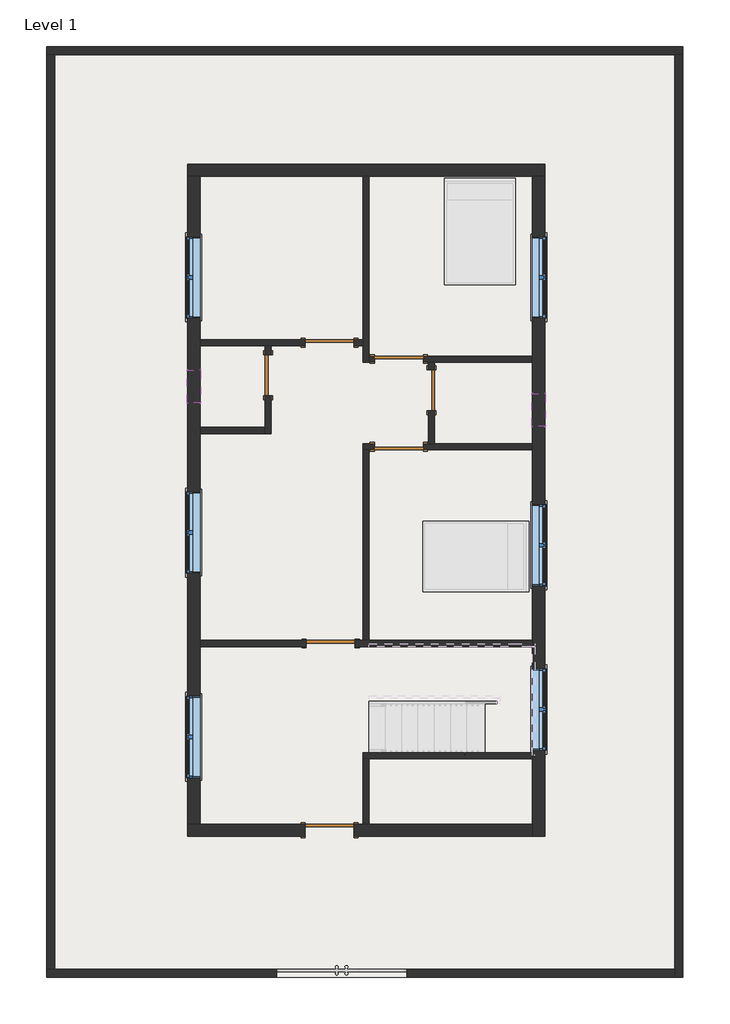
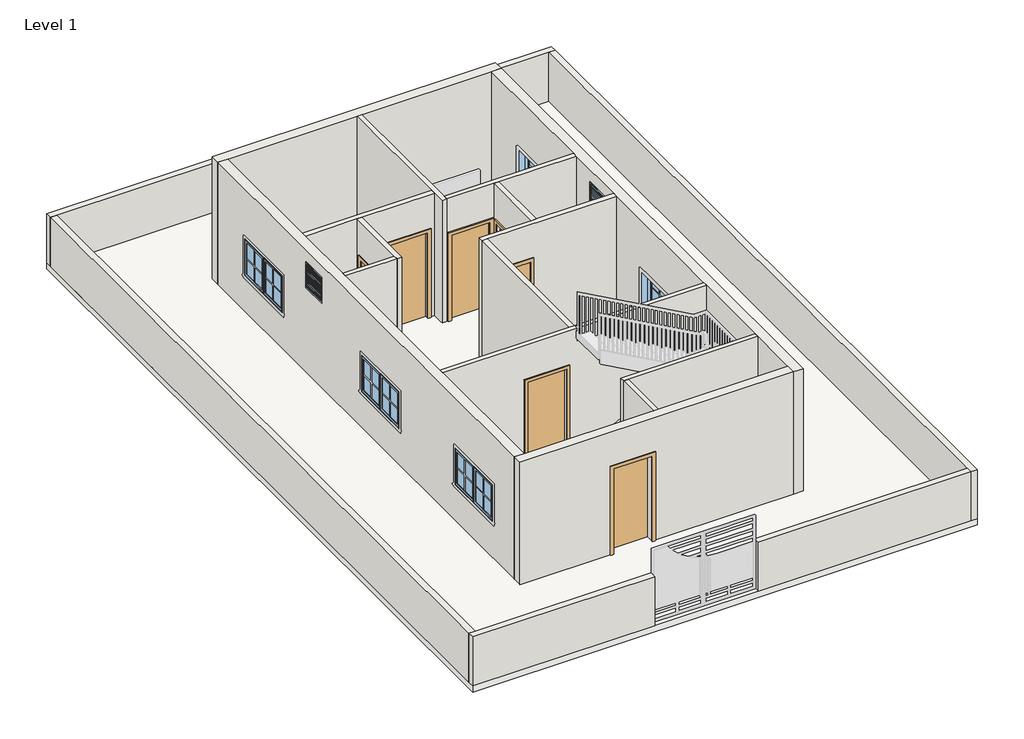
# One storey, part 1 of 3: 20 walls, 8 windows, 7 doors, 1 slab.
"""IFC4 building model written with IfcOpenShell, lengths in millimetres."""

from ifc_helpers import new_model, si_unit, frame, origin, origin_with_axes, place, context, project, spatial, polyline, outline, extrude, faceted_brep, transform, mapped, element, save
from components import door_78caadf7, door_214872d5, single_flush_door_3_e5f9f3c4, single_flush_door_3_305aa2a5, single_flush_door_3_0ca8825f, window_casement_double_win_5_c1d95f0f, window_f2d8fef0

model = new_model("IFC4")

# Units and contexts
model_context = context("Model", 3, world=origin())
ifc_project = project(units=[si_unit("LENGTHUNIT", "METRE", prefix="MILLI")], contexts=[model_context])

# Site, building, storey
site = spatial("IfcSite", under=ifc_project)
building = spatial("IfcBuilding", under=site)
storey = spatial("IfcBuildingStorey", under=building, Name="Level 1", Elevation=0.0)

# Doors
placement = place(None, origin())
door_shape = door_78caadf7(model_context)
element("IfcDoor", 1, ObjectType="Single-Flush : 2'6\"", at=placement, inside=storey, context=model_context, shape_type="MappedRepresentation", body=[
    mapped(door_shape, transform((-35.92188, 1946.24131, 0.0), x_axis=(0.0, 1.0, 0.0), y_axis=(-1.0, 0.0, 0.0), z_axis=(0.0, 0.0, 1.0))),
])
door_2_shape = door_214872d5(model_context)
element("IfcDoor", 2, ObjectType="Single-Flush : 2'6\"", at=placement, inside=storey, context=model_context, shape_type="MappedRepresentation", body=[
    mapped(door_2_shape, transform((-3083.92188, 2225.64131, 0.0), x_axis=(0.0, 1.0, 0.0), y_axis=(-1.0, 0.0, 0.0), z_axis=(0.0, 0.0, 1.0))),
])
single_flush_door_3_shape = single_flush_door_3_e5f9f3c4(model_context)
element("IfcDoor", 3, ObjectType="Single-Flush : DOOR 3'", at=placement, inside=storey, context=model_context, shape_type="MappedRepresentation", body=[
    mapped(single_flush_door_3_shape, transform((-1940.92188, 2835.24131, 0.0), x_axis=(1.0, 0.0, 0.0), y_axis=(0.0, 1.0, 0.0), z_axis=(0.0, 0.0, 1.0))),
])
element("IfcDoor", 4, ObjectType="Single-Flush : DOOR 3'", at=placement, inside=storey, context=model_context, shape_type="MappedRepresentation", body=[
    mapped(single_flush_door_3_shape, transform((-645.52188, 892.14131, 0.0), x_axis=(-1.0, 0.0, 0.0), y_axis=(0.0, -1.0, 0.0), z_axis=(0.0, 0.0, 1.0))),
])
element("IfcDoor", 5, ObjectType="Single-Flush : DOOR 3'", at=placement, inside=storey, context=model_context, shape_type="MappedRepresentation", body=[
    mapped(single_flush_door_3_shape, transform((-1915.52188, -2778.15869, 0.0), x_axis=(1.0, 0.0, 0.0), y_axis=(0.0, 1.0, 0.0), z_axis=(0.0, 0.0, 1.0))),
])
single_flush_door_3_2_shape = single_flush_door_3_305aa2a5(model_context)
element("IfcDoor", 6, ObjectType="Single-Flush : DOOR 3'", at=placement, inside=storey, context=model_context, shape_type="MappedRepresentation", body=[
    mapped(single_flush_door_3_2_shape, transform((-645.52188, 2530.44131, 0.0), x_axis=(-1.0, 0.0, 0.0), y_axis=(0.0, -1.0, 0.0), z_axis=(0.0, 0.0, 1.0))),
])
single_flush_door_3_3_shape = single_flush_door_3_0ca8825f(model_context)
element("IfcDoor", 7, ObjectType="Single-Flush : DOOR 3'", at=placement, inside=storey, context=model_context, shape_type="MappedRepresentation", body=[
    mapped(single_flush_door_3_3_shape, transform((-1940.92188, -6264.30869, 0.0), x_axis=(1.0, 0.0, 0.0), y_axis=(0.0, 1.0, 0.0), z_axis=(0.0, 0.0, 1.0))),
])

# Slab
element("IfcSlab", 8, ObjectType="FLOOR 6\"", at=placement, inside=storey, context=model_context, shape_type="SweptSolid", body=[
    extrude(outline(polyline([(4662.9483709, 8363.0499713), (4662.9483709, -9010.5500287), (-7224.2516291, -9010.5500287), (-7224.2516291, 8363.0499713), (4662.9483709, 8363.0499713)])), frame((0.0, 0.0, -152.4), z_axis=(0.0, 0.0, 1.0), x_axis=(1.0, 0.0, 0.0)), (0.0, 0.0, 1.0), 152.4),
])

# Walls
element("IfcWall", 9, ObjectType="CMD 6\"", at=placement, inside=storey, context=model_context, shape_type="Brep", body=[
    faceted_brep([(-7224.2516291, 8210.6499713, 0.0), (-7071.8516291, 8210.6499713, 0.0), (4510.5483709, 8210.6499713, 0.0), (4662.9483709, 8210.6499713, 0.0), (4662.9483709, 8210.6499713, 1219.2), (4510.5483709, 8210.6499713, 1219.2), (-7071.8516291, 8210.6499713, 1219.2), (-7224.2516291, 8210.6499713, 1219.2), (-7224.2516291, 8363.0499713, 0.0), (-7224.2516291, 8363.0499713, 1219.2), (4662.9483709, 8363.0499713, 1219.2), (4662.9483709, 8363.0499713, 0.0)], [[[0, 1, 2, 3, 4, 5, 6, 7]], [[8, 9, 10, 11]], [[3, 2, 1, 0, 8, 11]], [[7, 6, 5, 4, 10, 9]], [[4, 3, 11, 10]], [[0, 7, 9, 8]]]),
])
element("IfcWall", 10, ObjectType="CMD 6\"", at=placement, inside=storey, context=model_context, shape_type="Brep", body=[
    faceted_brep([(4510.5483709, 8210.6499713, 0.0), (4510.5483709, -8858.1500287, 0.0), (4510.5483709, -9010.5500287, 0.0), (4510.5483709, -9010.5500287, 1219.2), (4510.5483709, -8858.1500287, 1219.2), (4510.5483709, 8210.6499713, 1219.2), (4662.9483709, 8210.6499713, 0.0), (4662.9483709, 8210.6499713, 1219.2), (4662.9483709, -9010.5500287, 1219.2), (4662.9483709, -9010.5500287, 0.0)], [[[0, 1, 2, 3, 4, 5]], [[6, 7, 8, 9]], [[2, 1, 0, 6, 9]], [[5, 4, 3, 8, 7]], [[0, 5, 7, 6]], [[3, 2, 9, 8]]]),
])
element("IfcWall", 11, ObjectType="CMD 6\"", at=placement, inside=storey, context=model_context, shape_type="SweptSolid", body=[
    extrude(outline(polyline([(-493.12188, -8858.1500287), (4510.5483709, -8858.1500287), (4510.5483709, -9010.5500287), (-493.12188, -9010.5500287), (-493.12188, -8858.1500287)])), origin_with_axes(), (0.0, 0.0, 1.0), 1219.2),
])
element("IfcWall", 12, ObjectType="CMD 6\"", at=placement, inside=storey, context=model_context, shape_type="SweptSolid", body=[
    extrude(outline(polyline([(-7071.8516291, 8210.6499713), (-7071.8516291, -8858.1500287), (-7224.2516291, -8858.1500287), (-7224.2516291, 8210.6499713), (-7071.8516291, 8210.6499713)])), origin_with_axes(), (0.0, 0.0, 1.0), 1219.2),
])
element("IfcWall", 13, ObjectType="CMD 6\"", at=placement, inside=storey, context=model_context, shape_type="Brep", body=[
    faceted_brep([(-2931.52188, -8858.1500287, 0.0), (-7071.8516291, -8858.1500287, 0.0), (-7224.2516291, -8858.1500287, 0.0), (-7224.2516291, -8858.1500287, 1219.2), (-7071.8516291, -8858.1500287, 1219.2), (-2931.52188, -8858.1500287, 1219.2), (-2931.52188, -9010.5500287, 0.0), (-2931.52188, -9010.5500287, 1219.2), (-7224.2516291, -9010.5500287, 1219.2), (-7224.2516291, -9010.5500287, 0.0)], [[[0, 1, 2, 3, 4, 5]], [[6, 7, 8, 9]], [[2, 1, 0, 6, 9]], [[5, 4, 3, 8, 7]], [[0, 5, 7, 6]], [[3, 2, 9, 8]]]),
])
element("IfcWall", 14, ObjectType="WALL 4.5'", at=placement, inside=storey, context=model_context, shape_type="Brep", body=[
    faceted_brep([(-1312.27188, 5940.39131, 0.0), (-1312.27188, 2892.39131, 0.0), (-1312.27188, 2778.09131, 0.0), (-1312.27188, 2473.29131, 0.0), (-1312.27188, 2473.29131, 3048.0), (-1312.27188, 2778.09131, 3048.0), (-1312.27188, 2892.39131, 3048.0), (-1312.27188, 5940.39131, 3048.0), (-1197.97188, 5940.39131, 0.0), (-1197.97188, 5940.39131, 3048.0), (-1197.97188, 2587.59131, 3048.0), (-1197.97188, 2473.29131, 3048.0), (-1197.97188, 2473.29131, 0.0), (-1197.97188, 2587.59131, 0.0)], [[[0, 1, 2, 3, 4, 5, 6, 7]], [[8, 9, 10, 11, 12, 13]], [[3, 2, 1, 0, 8, 13, 12]], [[0, 7, 9, 8]], [[4, 3, 12, 11]], [[7, 6, 5, 4, 11, 10, 9]]]),
])
element("IfcWall", 15, ObjectType="WALL 4.5'", at=placement, inside=storey, context=model_context, shape_type="Brep", body=[
    faceted_brep([(-1197.97188, 2473.29131, 0.0), (-1102.72188, 2473.29131, 0.0), (-1102.72188, 2473.29131, 2133.6), (-188.32188, 2473.29131, 2133.6), (-188.32188, 2473.29131, 0.0), (-93.07188, 2473.29131, 0.0), (21.22812, 2473.29131, 0.0), (1850.02812, 2473.29131, 0.0), (1850.02812, 2473.29131, 3048.0), (21.22812, 2473.29131, 3048.0), (-93.07188, 2473.29131, 3048.0), (-1197.97188, 2473.29131, 3048.0), (-1102.72188, 2587.59131, 2133.6), (-1102.72188, 2587.59131, 0.0), (-1197.97188, 2587.59131, 0.0), (-1197.97188, 2587.59131, 3048.0), (1850.02812, 2587.59131, 3048.0), (1850.02812, 2587.59131, 0.0), (-188.32188, 2587.59131, 0.0), (-188.32188, 2587.59131, 2133.6)], [[[0, 1, 2, 3, 4, 5, 6, 7, 8, 9, 10, 11]], [[12, 13, 14, 15, 16, 17, 18, 19]], [[18, 17, 7, 6, 5, 4]], [[14, 13, 1, 0]], [[0, 11, 15, 14]], [[8, 7, 17, 16]], [[2, 1, 13, 12]], [[3, 2, 12, 19]], [[4, 3, 19, 18]], [[11, 10, 9, 8, 16, 15]]]),
])
element("IfcWall", 16, ObjectType="WALL 4.5'", at=placement, inside=storey, context=model_context, shape_type="Brep", body=[
    faceted_brep([(-1312.27188, 2892.39131, 0.0), (-1483.72188, 2892.39131, 0.0), (-1483.72188, 2892.39131, 2133.6), (-2398.12188, 2892.39131, 2133.6), (-2398.12188, 2892.39131, 0.0), (-4360.27188, 2892.39131, 0.0), (-4360.27188, 2892.39131, 3048.0), (-1312.27188, 2892.39131, 3048.0), (-1483.72188, 2778.09131, 2133.6), (-1483.72188, 2778.09131, 0.0), (-1312.27188, 2778.09131, 0.0), (-1312.27188, 2778.09131, 3048.0), (-3026.77188, 2778.09131, 3048.0), (-3141.07188, 2778.09131, 3048.0), (-4360.27188, 2778.09131, 3048.0), (-4360.27188, 2778.09131, 0.0), (-3141.07188, 2778.09131, 0.0), (-3026.77188, 2778.09131, 0.0), (-2398.12188, 2778.09131, 0.0), (-2398.12188, 2778.09131, 2133.6)], [[[0, 1, 2, 3, 4, 5, 6, 7]], [[8, 9, 10, 11, 12, 13, 14, 15, 16, 17, 18, 19]], [[10, 9, 1, 0]], [[18, 17, 16, 15, 5, 4]], [[6, 5, 15, 14]], [[0, 7, 11, 10]], [[2, 1, 9, 8]], [[3, 2, 8, 19]], [[4, 3, 19, 18]], [[7, 6, 14, 13, 12, 11]]]),
])
element("IfcWall", 17, ObjectType="WALL 4.5'", at=placement, inside=storey, context=model_context, shape_type="Brep", body=[
    faceted_brep([(-3141.07188, 2778.09131, 0.0), (-3141.07188, 2606.64131, 0.0), (-3141.07188, 2606.64131, 2133.6), (-3141.07188, 1844.64131, 2133.6), (-3141.07188, 1844.64131, 0.0), (-3141.07188, 1254.09131, 0.0), (-3141.07188, 1139.79131, 0.0), (-3141.07188, 1139.79131, 3048.0), (-3141.07188, 1254.09131, 3048.0), (-3141.07188, 2778.09131, 3048.0), (-3026.77188, 2606.64131, 2133.6), (-3026.77188, 2606.64131, 0.0), (-3026.77188, 2778.09131, 0.0), (-3026.77188, 2778.09131, 3048.0), (-3026.77188, 1139.79131, 3048.0), (-3026.77188, 1139.79131, 0.0), (-3026.77188, 1844.64131, 0.0), (-3026.77188, 1844.64131, 2133.6)], [[[0, 1, 2, 3, 4, 5, 6, 7, 8, 9]], [[10, 11, 12, 13, 14, 15, 16, 17]], [[16, 15, 6, 5, 4]], [[12, 11, 1, 0]], [[0, 9, 13, 12]], [[7, 6, 15, 14]], [[2, 1, 11, 10]], [[3, 2, 10, 17]], [[4, 3, 17, 16]], [[9, 8, 7, 14, 13]]]),
])
element("IfcWall", 18, ObjectType="WALL 4.5'", at=placement, inside=storey, context=model_context, shape_type="SweptSolid", body=[
    extrude(outline(polyline([(-4360.27188, 1254.09131), (-3141.07188, 1254.09131), (-3141.07188, 1139.79131), (-4360.27188, 1139.79131), (-4360.27188, 1254.09131)])), origin_with_axes(), (0.0, 0.0, 1.0), 3048.0),
])
element("IfcWall", 19, ObjectType="WALL 4.5'", at=placement, inside=storey, context=model_context, shape_type="SweptSolid", body=[
    extrude(outline(polyline([(2473.29131, 0.0), (2327.24131, 0.0), (2327.24131, 2133.6), (1565.24131, 2133.6), (1565.24131, 0.0), (949.29131, 0.0), (949.29131, 3048.0), (2473.29131, 3048.0), (2473.29131, 0.0)])), frame((-93.07188, 0.0, 0.0), z_axis=(1.0, 0.0, 0.0), x_axis=(0.0, 1.0, 0.0)), (0.0, 0.0, 1.0), 114.3),
])
element("IfcWall", 20, ObjectType="WALL 4.5'", at=placement, inside=storey, context=model_context, shape_type="Brep", body=[
    faceted_brep([(-1102.72188, 949.29131, 2133.6), (-1102.72188, 949.29131, 0.0), (-1312.27188, 949.29131, 0.0), (-1312.27188, 949.29131, 3048.0), (-93.07188, 949.29131, 3048.0), (21.22812, 949.29131, 3048.0), (1850.02812, 949.29131, 3048.0), (1850.02812, 949.29131, 0.0), (21.22812, 949.29131, 0.0), (-93.07188, 949.29131, 0.0), (-188.32188, 949.29131, 0.0), (-188.32188, 949.29131, 2133.6), (-1312.27188, 834.99131, 0.0), (-1197.97188, 834.99131, 0.0), (-1102.72188, 834.99131, 0.0), (-1102.72188, 834.99131, 2133.6), (-188.32188, 834.99131, 2133.6), (-188.32188, 834.99131, 0.0), (1850.02812, 834.99131, 0.0), (1850.02812, 834.99131, 3048.0), (-1197.97188, 834.99131, 3048.0), (-1312.27188, 834.99131, 3048.0)], [[[0, 1, 2, 3, 4, 5, 6, 7, 8, 9, 10, 11]], [[12, 13, 14, 15, 16, 17, 18, 19, 20, 21]], [[2, 1, 14, 13, 12]], [[10, 9, 8, 7, 18, 17]], [[7, 6, 19, 18]], [[3, 2, 12, 21]], [[15, 14, 1, 0]], [[16, 15, 0, 11]], [[17, 16, 11, 10]], [[6, 5, 4, 3, 21, 20, 19]]]),
])
element("IfcWall", 21, ObjectType="WALL 4.5'", at=placement, inside=storey, context=model_context, shape_type="SweptSolid", body=[
    extrude(outline(polyline([(-1312.27188, -2721.00869), (-1312.27188, 834.99131), (-1197.97188, 834.99131), (-1197.97188, -2721.00869), (-1312.27188, -2721.00869)])), origin_with_axes(), (0.0, 0.0, 1.0), 3048.0),
])
element("IfcWall", 22, ObjectType="WALL 4.5'", at=placement, inside=storey, context=model_context, shape_type="Brep", body=[
    faceted_brep([(1850.02812, -2721.00869, 0.0), (-1197.97188, -2721.00869, 0.0), (-1312.27188, -2721.00869, 0.0), (-1458.32188, -2721.00869, 0.0), (-1458.32188, -2721.00869, 2133.6), (-2372.72188, -2721.00869, 2133.6), (-2372.72188, -2721.00869, 0.0), (-4360.27188, -2721.00869, 0.0), (-4360.27188, -2721.00869, 3048.0), (-1312.27188, -2721.00869, 3048.0), (-1197.97188, -2721.00869, 3048.0), (1850.02812, -2721.00869, 3048.0), (-1458.32188, -2835.30869, 2133.6), (-1458.32188, -2835.30869, 0.0), (1850.02812, -2835.30869, 0.0), (1850.02812, -2835.30869, 3048.0), (-4360.27188, -2835.30869, 3048.0), (-4360.27188, -2835.30869, 0.0), (-2372.72188, -2835.30869, 0.0), (-2372.72188, -2835.30869, 2133.6)], [[[0, 1, 2, 3, 4, 5, 6, 7, 8, 9, 10, 11]], [[12, 13, 14, 15, 16, 17, 18, 19]], [[18, 17, 7, 6]], [[14, 13, 3, 2, 1, 0]], [[0, 11, 15, 14]], [[8, 7, 17, 16]], [[4, 3, 13, 12]], [[5, 4, 12, 19]], [[6, 5, 19, 18]], [[11, 10, 9, 8, 16, 15]]]),
])
element("IfcWall", 23, ObjectType="WALL 4.5'", at=placement, inside=storey, context=model_context, shape_type="Brep", body=[
    faceted_brep([(1850.02812, -4816.50869, 0.0), (-1312.27188, -4816.50869, 0.0), (-1312.27188, -4816.50869, 3048.0), (1850.02812, -4816.50869, 3048.0), (1850.02812, -4930.80869, 0.0), (1850.02812, -4930.80869, 3048.0), (-1197.97188, -4930.80869, 3048.0), (-1312.27188, -4930.80869, 3048.0), (-1312.27188, -4930.80869, 0.0), (-1197.97188, -4930.80869, 0.0)], [[[0, 1, 2, 3]], [[4, 5, 6, 7, 8, 9]], [[1, 0, 4, 9, 8]], [[0, 3, 5, 4]], [[2, 1, 8, 7]], [[3, 2, 7, 6, 5]]]),
])
element("IfcWall", 24, ObjectType="WALL 4.5'", at=placement, inside=storey, context=model_context, shape_type="SweptSolid", body=[
    extrude(outline(polyline([(-1312.27188, -6150.00869), (-1312.27188, -4930.80869), (-1197.97188, -4930.80869), (-1197.97188, -6150.00869), (-1312.27188, -6150.00869)])), origin_with_axes(), (0.0, 0.0, 1.0), 3048.0),
])
element("IfcWall", 25, ObjectType="WALL 9\"", at=placement, inside=storey, context=model_context, shape_type="Brep", body=[
    faceted_brep([(-4588.87188, 5940.39131, 0.0), (-4360.27188, 5940.39131, 0.0), (-1312.27188, 5940.39131, 0.0), (-1197.97188, 5940.39131, 0.0), (1850.02812, 5940.39131, 0.0), (2078.62812, 5940.39131, 0.0), (2078.62812, 5940.39131, 3048.0), (1850.02812, 5940.39131, 3048.0), (-1197.97188, 5940.39131, 3048.0), (-1312.27188, 5940.39131, 3048.0), (-4360.27188, 5940.39131, 3048.0), (-4588.87188, 5940.39131, 3048.0), (-4588.87188, 6168.99131, 0.0), (-4588.87188, 6168.99131, 3048.0), (2078.62812, 6168.99131, 3048.0), (2078.62812, 6168.99131, 0.0)], [[[0, 1, 2, 3, 4, 5, 6, 7, 8, 9, 10, 11]], [[12, 13, 14, 15]], [[5, 4, 3, 2, 1, 0, 12, 15]], [[6, 5, 15, 14]], [[0, 11, 13, 12]], [[11, 10, 9, 8, 7, 6, 14, 13]]]),
])
element("IfcWall", 26, ObjectType="WALL 9\"", at=placement, inside=storey, context=model_context, shape_type="Brep", body=[
    faceted_brep([(1850.02812, 5940.39131, 0.0), (1850.02812, 2587.59131, 0.0), (1850.02812, 2473.29131, 0.0), (1850.02812, 949.29131, 0.0), (1850.02812, 834.99131, 0.0), (1850.02812, -2721.00869, 0.0), (1850.02812, -2835.30869, 0.0), (1850.02812, -4816.50869, 0.0), (1850.02812, -4930.80869, 0.0), (1850.02812, -6150.00869, 0.0), (1850.02812, -6378.60869, 0.0), (1850.02812, -6378.60869, 3048.0), (1850.02812, -6150.00869, 3048.0), (1850.02812, -4930.80869, 3048.0), (1850.02812, -4816.50869, 3048.0), (1850.02812, -2835.30869, 3048.0), (1850.02812, -2721.00869, 3048.0), (1850.02812, 834.99131, 3048.0), (1850.02812, 949.29131, 3048.0), (1850.02812, 2473.29131, 3048.0), (1850.02812, 2587.59131, 3048.0), (1850.02812, 5940.39131, 3048.0), (1850.02812, -4772.05869, 1828.8), (1850.02812, -4772.05869, 914.4), (1850.02812, -3248.05869, 914.4), (1850.02812, -3248.05869, 1828.8), (1850.02812, 3292.44131, 1828.8), (1850.02812, 3292.44131, 914.4), (1850.02812, 4816.44131, 914.4), (1850.02812, 4816.44131, 1828.8), (1850.02812, -1705.00869, 1828.8), (1850.02812, -1705.00869, 914.4), (1850.02812, -181.00869, 914.4), (1850.02812, -181.00869, 1828.8), (1850.02812, 1273.14131, 2743.2), (1850.02812, 1273.14131, 2133.6), (1850.02812, 1882.74131, 2133.6), (1850.02812, 1882.74131, 2743.2), (2078.62812, 5940.39131, 0.0), (2078.62812, 5940.39131, 3048.0), (2078.62812, -6378.60869, 3048.0), (2078.62812, -6378.60869, 0.0), (2078.62812, -4772.05869, 1828.8), (2078.62812, -3248.05869, 1828.8), (2078.62812, -3248.05869, 914.4), (2078.62812, -4772.05869, 914.4), (2078.62812, 3292.44131, 1828.8), (2078.62812, 4816.44131, 1828.8), (2078.62812, 4816.44131, 914.4), (2078.62812, 3292.44131, 914.4), (2078.62812, -1705.00869, 1828.8), (2078.62812, -181.00869, 1828.8), (2078.62812, -181.00869, 914.4), (2078.62812, -1705.00869, 914.4), (2078.62812, 1273.14131, 2743.2), (2078.62812, 1882.74131, 2743.2), (2078.62812, 1882.74131, 2133.6), (2078.62812, 1273.14131, 2133.6)], [[[0, 1, 2, 3, 4, 5, 6, 7, 8, 9, 10, 11, 12, 13, 14, 15, 16, 17, 18, 19, 20, 21], [22, 23, 24, 25], [26, 27, 28, 29], [30, 31, 32, 33], [34, 35, 36, 37]], [[38, 39, 40, 41], [42, 43, 44, 45], [46, 47, 48, 49], [50, 51, 52, 53], [54, 55, 56, 57]], [[10, 9, 8, 7, 6, 5, 4, 3, 2, 1, 0, 38, 41]], [[0, 21, 39, 38]], [[11, 10, 41, 40]], [[23, 22, 42, 45]], [[24, 23, 45, 44]], [[25, 24, 44, 43]], [[22, 25, 43, 42]], [[27, 26, 46, 49]], [[28, 27, 49, 48]], [[29, 28, 48, 47]], [[26, 29, 47, 46]], [[31, 30, 50, 53]], [[32, 31, 53, 52]], [[33, 32, 52, 51]], [[30, 33, 51, 50]], [[35, 34, 54, 57]], [[36, 35, 57, 56]], [[37, 36, 56, 55]], [[34, 37, 55, 54]], [[21, 20, 19, 18, 17, 16, 15, 14, 13, 12, 11, 40, 39]]]),
])
element("IfcWall", 27, ObjectType="WALL 9\"", at=placement, inside=storey, context=model_context, shape_type="Brep", body=[
    faceted_brep([(1850.02812, -6150.00869, 0.0), (-1197.97188, -6150.00869, 0.0), (-1312.27188, -6150.00869, 0.0), (-1483.72188, -6150.00869, 0.0), (-1483.72188, -6150.00869, 2133.6), (-2398.12188, -6150.00869, 2133.6), (-2398.12188, -6150.00869, 0.0), (-4360.27188, -6150.00869, 0.0), (-4588.87188, -6150.00869, 0.0), (-4588.87188, -6150.00869, 3048.0), (-4360.27188, -6150.00869, 3048.0), (-1312.27188, -6150.00869, 3048.0), (-1197.97188, -6150.00869, 3048.0), (1850.02812, -6150.00869, 3048.0), (-1483.72188, -6378.60869, 2133.6), (-1483.72188, -6378.60869, 0.0), (1850.02812, -6378.60869, 0.0), (1850.02812, -6378.60869, 3048.0), (-4588.87188, -6378.60869, 3048.0), (-4588.87188, -6378.60869, 0.0), (-2398.12188, -6378.60869, 0.0), (-2398.12188, -6378.60869, 2133.6)], [[[0, 1, 2, 3, 4, 5, 6, 7, 8, 9, 10, 11, 12, 13]], [[14, 15, 16, 17, 18, 19, 20, 21]], [[20, 19, 8, 7, 6]], [[16, 15, 3, 2, 1, 0]], [[0, 13, 17, 16]], [[9, 8, 19, 18]], [[4, 3, 15, 14]], [[5, 4, 14, 21]], [[6, 5, 21, 20]], [[13, 12, 11, 10, 9, 18, 17]]]),
])
element("IfcWall", 28, ObjectType="WALL 9\"", at=placement, inside=storey, context=model_context, shape_type="Brep", body=[
    faceted_brep([(-4360.27188, -6150.00869, 0.0), (-4360.27188, -2835.30869, 0.0), (-4360.27188, -2721.00869, 0.0), (-4360.27188, 1139.79131, 0.0), (-4360.27188, 1254.09131, 0.0), (-4360.27188, 2778.09131, 0.0), (-4360.27188, 2892.39131, 0.0), (-4360.27188, 5940.39131, 0.0), (-4360.27188, 5940.39131, 3048.0), (-4360.27188, 2892.39131, 3048.0), (-4360.27188, 2778.09131, 3048.0), (-4360.27188, 1254.09131, 3048.0), (-4360.27188, 1139.79131, 3048.0), (-4360.27188, -2721.00869, 3048.0), (-4360.27188, -2835.30869, 3048.0), (-4360.27188, -6150.00869, 3048.0), (-4360.27188, 4816.44131, 1828.8), (-4360.27188, 4816.44131, 914.4), (-4360.27188, 3292.44131, 914.4), (-4360.27188, 3292.44131, 1828.8), (-4360.27188, 53.94131, 1828.8), (-4360.27188, 53.94131, 914.4), (-4360.27188, -1470.05869, 914.4), (-4360.27188, -1470.05869, 1828.8), (-4360.27188, -3759.23369, 1828.8), (-4360.27188, -3759.23369, 914.4), (-4360.27188, -5283.23369, 914.4), (-4360.27188, -5283.23369, 1828.8), (-4360.27188, 1711.29131, 2743.2), (-4360.27188, 2320.89131, 2743.2), (-4360.27188, 2320.89131, 2133.6), (-4360.27188, 1711.29131, 2133.6), (-4588.87188, -6150.00869, 0.0), (-4588.87188, -6150.00869, 3048.0), (-4588.87188, 5940.39131, 3048.0), (-4588.87188, 5940.39131, 0.0), (-4588.87188, 4816.44131, 1828.8), (-4588.87188, 3292.44131, 1828.8), (-4588.87188, 3292.44131, 914.4), (-4588.87188, 4816.44131, 914.4), (-4588.87188, 53.94131, 1828.8), (-4588.87188, -1470.05869, 1828.8), (-4588.87188, -1470.05869, 914.4), (-4588.87188, 53.94131, 914.4), (-4588.87188, -3759.23369, 1828.8), (-4588.87188, -5283.23369, 1828.8), (-4588.87188, -5283.23369, 914.4), (-4588.87188, -3759.23369, 914.4), (-4588.87188, 1711.29131, 2743.2), (-4588.87188, 1711.29131, 2133.6), (-4588.87188, 2320.89131, 2133.6), (-4588.87188, 2320.89131, 2743.2)], [[[0, 1, 2, 3, 4, 5, 6, 7, 8, 9, 10, 11, 12, 13, 14, 15], [16, 17, 18, 19], [20, 21, 22, 23], [24, 25, 26, 27], [28, 29, 30, 31]], [[32, 33, 34, 35], [36, 37, 38, 39], [40, 41, 42, 43], [44, 45, 46, 47], [48, 49, 50, 51]], [[7, 6, 5, 4, 3, 2, 1, 0, 32, 35]], [[8, 7, 35, 34]], [[0, 15, 33, 32]], [[17, 16, 36, 39]], [[18, 17, 39, 38]], [[19, 18, 38, 37]], [[16, 19, 37, 36]], [[21, 20, 40, 43]], [[22, 21, 43, 42]], [[23, 22, 42, 41]], [[20, 23, 41, 40]], [[25, 24, 44, 47]], [[26, 25, 47, 46]], [[27, 26, 46, 45]], [[24, 27, 45, 44]], [[49, 48, 28, 31]], [[50, 49, 31, 30]], [[51, 50, 30, 29]], [[48, 51, 29, 28]], [[15, 14, 13, 12, 11, 10, 9, 8, 34, 33]]]),
])

# Windows
window_casement_double_win_5_shape = window_casement_double_win_5_c1d95f0f(model_context)
element("IfcWindow", 29, ObjectType="Window-Casement-Double : WIN 5'", at=placement, inside=storey, context=model_context, shape_type="MappedRepresentation", body=[
    mapped(window_casement_double_win_5_shape, transform((-4474.57188, 4054.44131, 0.0), x_axis=(0.0, 1.0, 0.0), y_axis=(-1.0, 0.0, 0.0), z_axis=(0.0, 0.0, 1.0))),
])
element("IfcWindow", 30, ObjectType="Window-Casement-Double : WIN 5'", at=placement, inside=storey, context=model_context, shape_type="MappedRepresentation", body=[
    mapped(window_casement_double_win_5_shape, transform((-4474.57188, -708.05869, 0.0), x_axis=(0.0, 1.0, 0.0), y_axis=(-1.0, 0.0, 0.0), z_axis=(0.0, 0.0, 1.0))),
])
element("IfcWindow", 31, ObjectType="Window-Casement-Double : WIN 5'", at=placement, inside=storey, context=model_context, shape_type="MappedRepresentation", body=[
    mapped(window_casement_double_win_5_shape, transform((-4474.57188, -4521.23369, 0.0), x_axis=(0.0, 1.0, 0.0), y_axis=(-1.0, 0.0, 0.0), z_axis=(0.0, 0.0, 1.0))),
])
element("IfcWindow", 32, ObjectType="Window-Casement-Double : WIN 5'", at=placement, inside=storey, context=model_context, shape_type="MappedRepresentation", body=[
    mapped(window_casement_double_win_5_shape, transform((1964.32812, -4010.05869, 0.0), x_axis=(0.0, -1.0, 0.0), y_axis=(1.0, 0.0, 0.0), z_axis=(0.0, 0.0, 1.0))),
])
element("IfcWindow", 33, ObjectType="Window-Casement-Double : WIN 5'", at=placement, inside=storey, context=model_context, shape_type="MappedRepresentation", body=[
    mapped(window_casement_double_win_5_shape, transform((1964.32812, 4054.44131, 0.0), x_axis=(0.0, -1.0, 0.0), y_axis=(1.0, 0.0, 0.0), z_axis=(0.0, 0.0, 1.0))),
])
element("IfcWindow", 34, ObjectType="Window-Casement-Double : WIN 5'", at=placement, inside=storey, context=model_context, shape_type="MappedRepresentation", body=[
    mapped(window_casement_double_win_5_shape, transform((1964.32812, -943.00869, 0.0), x_axis=(0.0, -1.0, 0.0), y_axis=(1.0, 0.0, 0.0), z_axis=(0.0, 0.0, 1.0))),
])
window_shape = window_f2d8fef0(model_context)
element("IfcWindow", 35, ObjectType="Window-Louvers : 24\" x 24\"", at=placement, inside=storey, context=model_context, shape_type="MappedRepresentation", body=[
    mapped(window_shape, transform((1957.97812, 1577.94131, 1219.2), x_axis=(0.0, 1.0, 0.0), y_axis=(-1.0, 0.0, 0.0), z_axis=(0.0, 0.0, 1.0))),
])
element("IfcWindow", 36, ObjectType="Window-Louvers : 24\" x 24\"", at=placement, inside=storey, context=model_context, shape_type="MappedRepresentation", body=[
    mapped(window_shape, transform((-4480.92188, 2016.09131, 1219.2), x_axis=(0.0, 1.0, 0.0), y_axis=(-1.0, 0.0, 0.0), z_axis=(0.0, 0.0, 1.0))),
])

save(model, "model.ifc")

# Revit data of these elements
# Type "Single-Flush : 2'6\""
#   Type Mark = "9"
#   Construction Type Id = "MDOOR"
#   Assembly Code = "C1020"
#   Analytic Construction = "Metal"
#   Thickness = 0' - 2"
#   Heat Transfer Coefficient (U) = 0.651978 BTU/(h·ft²·°F)
#   Height = 7' - 0"
#   Trim Projection Ext = 0' - 1"
#   Trim Projection Int = 0' - 1"
#   Trim Width = 0' - 3"
#   Width = 2' - 6"
#   Define Thermal Properties by = 1
#   Door Material = Door - Panel
#   Frame Material = Door - Frame
#   Visual Light Transmittance = 0
#   Solar Heat Gain Coefficient = 0
#   Function = (empty or 0)
#   Wall Closure = (empty or 0)
# Type "Single-Flush : DOOR 3'"
#   Type Mark = "8"
#   Construction Type Id = "MDOOR"
#   Assembly Code = "C1020"
#   Analytic Construction = "Metal"
#   Thickness = 0' - 2"
#   Heat Transfer Coefficient (U) = 0.651978 BTU/(h·ft²·°F)
#   Height = 7' - 0"
#   Trim Projection Ext = 0' - 1"
#   Trim Projection Int = 0' - 1"
#   Trim Width = 0' - 3"
#   Width = 3' - 0"
#   Define Thermal Properties by = 1
#   Door Material = Door - Panel
#   Frame Material = Door - Frame
#   Visual Light Transmittance = 0
#   Solar Heat Gain Coefficient = 0
#   Function = (empty or 0)
#   Wall Closure = (empty or 0)
# Type "FLOOR 6\""
#   Assembly Code = "B1010"
#   Function = 0
#   Layers, outside or top first: 0' - 6" no material (function 1)
# Type "CMD 6\""
#   Assembly Code = "B2010"
#   Layers, outside or top first: 0' - 6" no material (function 1)
# Type "WALL 4.5'"
#   Assembly Code = "B2010"
#   Layers, outside or top first: 0' - 4 1/2" no material (function 1)
# Type "WALL 9\""
#   Assembly Code = "B2010"
#   Layers, outside or top first: 0' - 9" no material (function 1)
# Type "Window-Casement-Double : WIN 5'"
#   Type Mark = "18"
#   Fire Rating = "0.5h"
#   Assembly Code = "B2020100"
#   Analytic Construction = "Double glazing - domestic"
#   Frame Extension [instance default] = 0' - 0 1/4"
#   Window Inset [instance default] = 0' - 0"
#   Wall Thickness [instance default] = 0' - 6"
#   Interior Wall Closure [instance default] = 0' - 2 1/4"
#   Half Width = 2' - 6"
#   Visual Light Transmittance = 0.81
#   Thermal Resistance (R) = 1.8146 (h·ft²·°F)/BTU
#   Solar Heat Gain Coefficient = 0.76
#   Rough Width = 5' - 0 1/2"
#   Rough Height = 3' - 0 1/2"
#   Height = 3' - 0"
#   Heat Transfer Coefficient (U) = 0.5511 BTU/(h·ft²·°F)
#   Exterior Wall Closure [instance default] = 0' - 1 1/4"
#   Extension Jamb [instance default] = 0' - 2 1/4"
#   Default Sill Height = 3' - 0"
#   Width = 5' - 0"
#   Muntin Visibility = yes
#   Interior Trim Visibility [instance default] = yes
#   Exterior Trim Visibility [instance default] = yes
#   Extension Jamb Visibility [instance default] = yes
#   Interior Trim Material = Wood - Stained
#   Muntin Pattern = Muntin Pattern_2x2 : Muntin Pattern_2x2
#   Interior Trim = Trim-Window-Interior-Flat : Picture Frame
#   Interior Frame Material = Wood - Stained
#   Glass Panel Material = Glass
#   Exterior Trim Material = Clad - White
#   Exterior Trim = Trim-Window-Exterior-Flat : with Sill
#   Exterior Frame Material = Clad - White
#   Wall Closure = (empty or 0)
# Type "Window-Louvers : 24\" x 24\""
#   Type Mark = "19"
#   Construction Type Id = "GSP4R"
#   Assembly Code = "B20"
#   Analytic Construction = "1/8 in Pilkington single glazing"
#   Visual Light Transmittance = 0.9
#   Thermal Resistance (R) = 1.53941 (h·ft²·°F)/BTU
#   Solar Heat Gain Coefficient = 0.78
#   Max Height = 1' - 11.74264"
#   Height = 2' - 0"
#   Heat Transfer Coefficient (U) = 0.6496 BTU/(h·ft²·°F)
#   Blade Width [instance default] = 1' - 10 1/2"
#   Blade Vertical Thickness = 0' - 0.35355"
#   Blade Thickness = 0' - 0 1/4"
#   Blade Spacing = 0' - 1 1/2"
#   Blade Height = 0' - 1.85355"
#   Blade Depth = 0' - 3"
#   Blade Angle = 45.00°
#   Default Sill Height = 3' - 0"
#   Trim Projection_Exterior = 0' - 0 1/2"
#   Trim Projection_Interior = 0' - 0 1/2"
#   Trim Width_Exterior = 0' - 1 1/2"
#   Trim Width_Interior = 0' - 1 1/2"
#   Width = 2' - 0"
#   Max Blade Count = 12
#   Define Thermal Properties by = 1
#   Blade Count = 12
#   Frame Material = Birch
#   Louver Material = Birch
#   Trim Exterior Material = Birch
#   Trim Interior Material = Birch
#   Wall Closure = (empty or 0)
# Elements 1, 2 (IfcDoor, "Single-Flush : 2'6\"")
#   Phase Created = New Construction
#   Materials on its faces: "Door - Frame", "Door - Panel"
# Elements 3, 4, 5, 6, 7 (IfcDoor, "Single-Flush : DOOR 3'")
#   Phase Created = New Construction
#   Materials on its faces: "Door - Frame", "Door - Panel"
# Element 8 (IfcSlab, "FLOOR 6\"")
#   Height Offset From Level = 0' - 0"
#   Phase Created = New Construction
#   Materials on its faces: "Parking Stripe", "Default Floor", "Wood - Stained"
# Elements 9, 10, 11 (IfcWall, "CMD 6\"")
#   Top Offset = 0' - 0"
#   Base Offset = 0' - 0"
#   Unconnected Height = 4' - 0"
#   wall height = 4' - 0"
#   Phase Created = New Construction
#   Base Constraint = Level 1
#   Materials on its faces: "Clad - White", "Default Wall", "Parking Stripe"
# Element 12 (IfcWall, "CMD 6\"")
#   Top Offset = 0' - 0"
#   Base Offset = 0' - 0"
#   Unconnected Height = 4' - 0"
#   wall height = 4' - 0"
#   Phase Created = New Construction
#   Base Constraint = Level 1
#   Materials on its faces: "Default Wall", "Clad - White", "Parking Stripe"
# Element 13 (IfcWall, "CMD 6\"")
#   Top Offset = 0' - 0"
#   Base Offset = 0' - 0"
#   Unconnected Height = 4' - 0"
#   wall height = 4' - 0"
#   Phase Created = New Construction
#   Base Constraint = Level 1
#   Materials on its faces: "Clad - White", "Parking Stripe", "Default Wall"
# Elements 14, 15, 16, 17, 18, 19, 20, 21, 22, 23, 24 (IfcWall, "WALL 4.5'")
#   Top Offset = 0' - 0"
#   Base Offset = 0' - 0"
#   Unconnected Height = 10' - 0"
#   wall height = 10' - 0"
#   Phase Created = New Construction
#   Base Constraint = Level 1
#   Materials on its faces: "Default Wall"
# Elements 25, 26, 27, 28 (IfcWall, "WALL 9\"")
#   Top Offset = 0' - 0"
#   Base Offset = 0' - 0"
#   Unconnected Height = 10' - 0"
#   wall height = 10' - 0"
#   Phase Created = New Construction
#   Base Constraint = Level 1
#   Materials on its faces: "Default Wall", "Copper"
# Element 29 (IfcWindow, "Window-Casement-Double : WIN 5'")
#   Mark = "1"
#   Window Inset = 0' - 0"
#   Interior Wall Closure = 0' - 2 1/4"
#   Frame Extension = 0' - 0 1/4"
#   Exterior Wall Closure = 0' - 1 1/4"
#   Interior Trim Visibility = yes
#   Exterior Trim Visibility = yes
#   Phase Created = New Construction
#   Materials on its faces: "Wood - Stained", "Glass", "Clad - White"
# Element 30 (IfcWindow, "Window-Casement-Double : WIN 5'")
#   Mark = "2"
#   Window Inset = 0' - 0"
#   Interior Wall Closure = 0' - 2 1/4"
#   Frame Extension = 0' - 0 1/4"
#   Exterior Wall Closure = 0' - 1 1/4"
#   Interior Trim Visibility = yes
#   Exterior Trim Visibility = yes
#   Phase Created = New Construction
#   Materials on its faces: "Wood - Stained", "Glass", "Clad - White"
# Element 31 (IfcWindow, "Window-Casement-Double : WIN 5'")
#   Mark = "3"
#   Window Inset = 0' - 0"
#   Interior Wall Closure = 0' - 2 1/4"
#   Frame Extension = 0' - 0 1/4"
#   Exterior Wall Closure = 0' - 1 1/4"
#   Interior Trim Visibility = yes
#   Exterior Trim Visibility = yes
#   Phase Created = New Construction
#   Materials on its faces: "Wood - Stained", "Glass", "Clad - White"
# Element 32 (IfcWindow, "Window-Casement-Double : WIN 5'")
#   Mark = "4"
#   Window Inset = 0' - 0"
#   Interior Wall Closure = 0' - 2 1/4"
#   Frame Extension = 0' - 0 1/4"
#   Exterior Wall Closure = 0' - 1 1/4"
#   Interior Trim Visibility = yes
#   Exterior Trim Visibility = yes
#   Phase Created = New Construction
#   Materials on its faces: "Wood - Stained", "Glass", "Clad - White"
# Element 33 (IfcWindow, "Window-Casement-Double : WIN 5'")
#   Mark = "5"
#   Window Inset = 0' - 0"
#   Interior Wall Closure = 0' - 2 1/4"
#   Frame Extension = 0' - 0 1/4"
#   Exterior Wall Closure = 0' - 1 1/4"
#   Interior Trim Visibility = yes
#   Exterior Trim Visibility = yes
#   Phase Created = New Construction
#   Materials on its faces: "Wood - Stained", "Glass", "Clad - White"
# Element 34 (IfcWindow, "Window-Casement-Double : WIN 5'")
#   Mark = "6"
#   Window Inset = 0' - 0"
#   Interior Wall Closure = 0' - 2 1/4"
#   Frame Extension = 0' - 0 1/4"
#   Exterior Wall Closure = 0' - 1 1/4"
#   Interior Trim Visibility = yes
#   Exterior Trim Visibility = yes
#   Phase Created = New Construction
#   Materials on its faces: "Wood - Stained", "Glass", "Clad - White"
# Element 35 (IfcWindow, "Window-Louvers : 24\" x 24\"")
#   Mark = "7"
#   Blade Width = 1' - 10 1/2"
#   Phase Created = New Construction
#   Materials on its faces: "Birch"
# Element 36 (IfcWindow, "Window-Louvers : 24\" x 24\"")
#   Mark = "8"
#   Blade Width = 1' - 10 1/2"
#   Phase Created = New Construction
#   Materials on its faces: "Birch"
# Materials
#   "Door - Panel": class "Wood", colour RGB 210 159 95, transparency 0, Cost = 0
#   "Door - Frame": colour RGB 118 70 51, transparency 0, Cost = 0
#   "Wood - Stained": class "Wood", colour RGB 224 178 126, transparency 0, Cost = 0
#   "Glass": class "Glass", colour RGB 0 128 192, transparency 0.75, Description = "Soda Lime Glass", Cost = 0
#   "Clad - White": class "Wood", colour RGB 242 242 238, transparency 0, Cost = 0
#   "Birch": class "Wood", colour RGB 224 178 126, transparency 0, Description = "Betula Alleghaniensis", Cost = 0
#   "Parking Stripe": class "Paint", colour RGB 250 250 91, transparency 0, Cost = 0
#   "Default Floor": colour RGB 128 128 128, transparency 0, Cost = 0
#   "Default Wall": colour RGB 128 128 128, transparency 0, Cost = 0
#   "Copper": class "Metal", colour RGB 0 0 0, transparency 0, Description = "Copper, matte finish", Cost = 0
